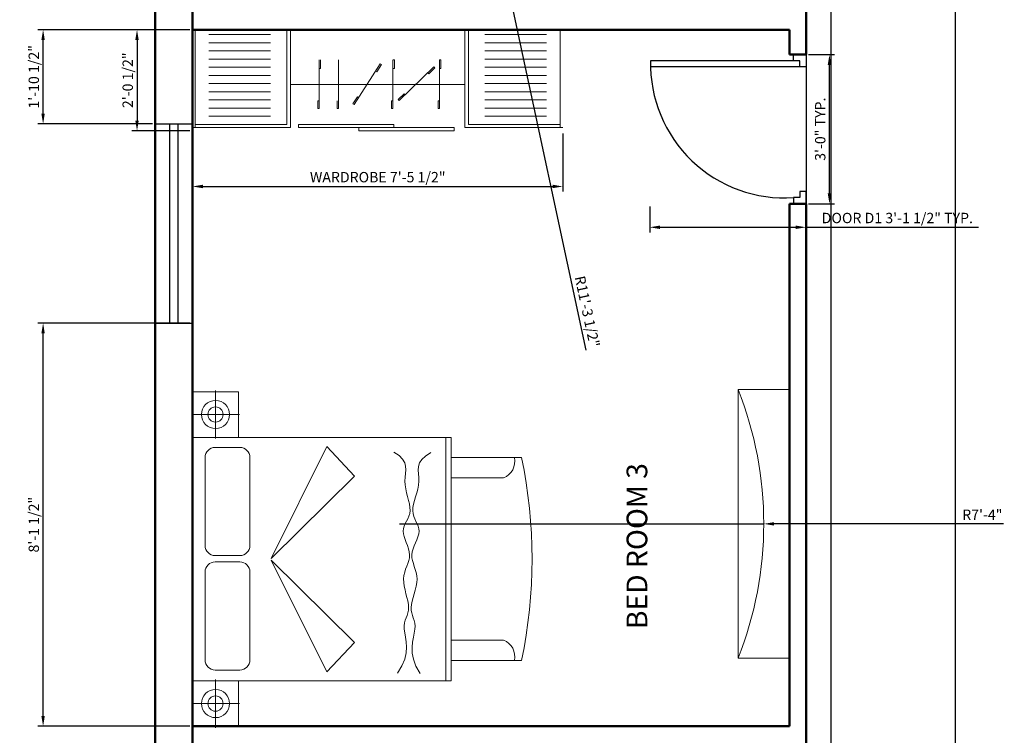
# Model space of a CAD drawing. Units: inches. Extents: x 1905 to 2315, y 3232 to 3824.
# Tile 2 of 8: x 1905 to 2143, y 3442 to 3615. Entities that reach past the tile are written whole.
import ezdxf

# ---------------------------------------------------------------- set-up
doc = ezdxf.new("R2010")
doc.units = ezdxf.units.IN
for name, color, linetype, lineweight in [('A-ANNO-DIMS', 2, 'Continuous', 18), ('A-AREA-IDEN', 7, 'Continuous', 25), ('A-FLOR-CABT', 8, 'Continuous', 18), ('A-FURN', 8, 'Continuous', 18), ('door', 1, 'Continuous', 25), ('TV', 221, 'Continuous', 18), ('wall', 2, 'Continuous', 50), ('WINDOW', 60, 'Continuous', 25)]:
    doc.layers.add(name, color=color, linetype=linetype, lineweight=lineweight)
doc.styles.get("Standard").update_dxf_attribs({"font": 'arial.ttf'})
doc.dimstyles.new('ISO-25', dxfattribs={"dimtxt": 2.5, "dimasz": 2.5, "dimexe": 1.25, "dimexo": 0.625, "dimtad": 1, "dimdec": 1, "dimlunit": 3, "dimtxsty": 'Standard', "dimcen": 2.5, "dimadec": 0, "dimazin": 0, "dimtfac": 1, "dimtdec": 1, "dimtmove": 0, "dimatfit": 3, "dimfxl": 1, "dimarcsym": 0})

# ---------------------------------------------------------------- blocks, each defined once
blk = doc.blocks.new('A$C4F543DC7')
for p, q in [((0.0134, 3.35, -0.1688), (3.3134, 3.35, -0.1688)), ((0.4634, 3.35, -0.1688), (0.0134, 3.35, -0.1688)), ((0.0134, 2.896, -0.1688), (0.0134, 3.35, -0.1688)), ((0.0134, 3.35, -0.1688), (0.0134, 2.896, -0.1688)), ((0.2381, 3.1233, -0.4388), (0.2381, 3.3614, -0.4388)), ((0.4634, 3.35, -0.1688), (0.4634, 0.8, -0.1688)), ((2.8634, 3.35, -0.1688), (0.4634, 3.35, -0.1688)), ((0.4634, 2.896, -0.1688), (0.4634, 3.35, -0.1688)), ((2.8634, 0.8, -0.1688), (2.8634, 3.35, -0.1688)), ((2.8634, 3.35, -0.1688), (3.3134, 3.35, -0.1688)), ((2.8634, 2.896, -0.1688), (2.8634, 3.35, -0.1688)), ((3.0888, 3.1233, -0.4388), (3.0888, 3.3614, -0.4388)), ((3.3134, 3.35, -0.1688), (3.3134, 2.896, -0.1688)), ((3.3134, 3.35, -0.1688), (3.3134, 2.896, -0.1688)), ((1.5354, 3.226, -0.1688), (0.6684, 3.226, -0.1688)), ((2.6644, 3.226, -0.1688), (1.7974, 3.226, -0.1688)), ((0.2381, 3.1233, -0.4388), (0, 3.1233, -0.4388)), ((0.2381, 3.1233, -0.4388), (0.4762, 3.1233, -0.4388)), ((0.2381, 3.1233, -0.4388), (0.2381, 2.8852, -0.4388)), ((0.5684, 3.126, -0.1688), (0.5684, 2.884, -0.1688)), ((1.6354, 2.884, -0.1688), (1.6354, 3.126, -0.1688)), ((1.6974, 3.126, -0.1688), (1.6974, 2.884, -0.1688)), ((2.7644, 2.884, -0.1688), (2.7644, 3.126, -0.1688)), ((3.0888, 3.1233, -0.4388), (2.8507, 3.1233, -0.4388)), ((3.0888, 3.1233, -0.4388), (3.0888, 2.8852, -0.4388)), ((3.0888, 3.1233, -0.4388), (3.3269, 3.1233, -0.4388)), ((0.4634, 2.896, -0.1688), (0.0134, 2.896, -0.1688)), ((0.0134, 2.896, -0.1688), (0.4634, 2.896, -0.1688)), ((0.4634, 0.8, -0.1688), (0.4634, 2.896, -0.1688)), ((2.8634, 2.896, -0.1688), (2.8634, 0.8, -0.1688)), ((3.3134, 2.896, -0.1688), (2.8634, 2.896, -0.1688)), ((3.3134, 2.896, -0.1688), (2.8634, 2.896, -0.1688)), ((0.6684, 2.784, -0.1688), (1.5354, 2.784, -0.1688)), ((1.7974, 2.784, -0.1688), (2.6644, 2.784, -0.1688)), ((1.6534, 2.573, -0.1688), (0.5504, 2.025, -0.1688)), ((0.8414, 1.752, -0.1688), (1.6534, 2.573, -0.1688)), ((2.4814, 1.752, -0.1688), (1.6694, 2.573, -0.1688)), ((1.6694, 2.573, -0.1688), (2.7724, 2.025, -0.1688)), ((0.5504, 2.025, -0.1688), (0.8414, 1.752, -0.1688)), ((2.7724, 2.025, -0.1688), (2.4814, 1.752, -0.1688)), ((2.683, 1.312, -0.1688), (2.7182, 1.3641, -0.1688)), ((0.5369, 1.3267, -0.1688), (0.6088, 1.2835, -0.1688)), ((0.6088, 1.2835, -0.1688), (0.6756, 1.2566, -0.1688)), ((1.3963, 1.2612, -0.1688), (1.4328, 1.2664, -0.1688)), ((1.4328, 1.2664, -0.1688), (1.4679, 1.2677, -0.1688)), ((1.4679, 1.2677, -0.1688), (1.501, 1.2643, -0.1688)), ((1.501, 1.2643, -0.1688), (1.5324, 1.257, -0.1688)), ((1.8557, 1.2531, -0.1688), (1.8849, 1.263, -0.1688)), ((1.8849, 1.263, -0.1688), (1.913, 1.2698, -0.1688)), ((1.913, 1.2698, -0.1688), (1.9397, 1.2722, -0.1688)), ((1.9397, 1.2722, -0.1688), (1.9649, 1.2692, -0.1688)), ((1.9649, 1.2692, -0.1688), (1.989, 1.2617, -0.1688)), ((2.6129, 1.257, -0.1688), (2.6479, 1.2774, -0.1688)), ((2.6479, 1.2774, -0.1688), (2.683, 1.312, -0.1688)), ((0.6067, 1.1458, -0.1688), (0.6743, 1.1706, -0.1688)), ((0.6743, 1.1706, -0.1688), (0.7364, 1.1825, -0.1688)), ((0.6756, 1.2566, -0.1688), (0.7373, 1.2428, -0.1688)), ((0.7364, 1.1825, -0.1688), (0.7931, 1.1846, -0.1688)), ((0.7373, 1.2428, -0.1688), (0.794, 1.239, -0.1688)), ((0.7931, 1.1846, -0.1688), (0.8447, 1.1799, -0.1688)), ((0.794, 1.239, -0.1688), (0.8457, 1.242, -0.1688)), ((0.8447, 1.1799, -0.1688), (0.8913, 1.1716, -0.1688)), ((0.8457, 1.242, -0.1688), (0.8925, 1.2489, -0.1688)), ((0.8913, 1.1716, -0.1688), (0.9331, 1.1628, -0.1688)), ((0.8925, 1.2489, -0.1688), (0.9345, 1.2564, -0.1688)), ((0.9345, 1.2564, -0.1688), (0.9718, 1.2615, -0.1688)), ((0.9718, 1.2615, -0.1688), (1.0044, 1.2617, -0.1688)), ((1.0044, 1.2617, -0.1688), (1.0334, 1.2578, -0.1688)), ((1.0334, 1.2578, -0.1688), (1.0597, 1.2509, -0.1688)), ((1.0583, 1.1642, -0.1688), (1.0831, 1.172, -0.1688)), ((1.0597, 1.2509, -0.1688), (1.0842, 1.2424, -0.1688)), ((1.0831, 1.172, -0.1688), (1.1072, 1.18, -0.1688)), ((1.0842, 1.2424, -0.1688), (1.1081, 1.2336, -0.1688)), ((1.1072, 1.18, -0.1688), (1.1316, 1.1872, -0.1688)), ((1.1081, 1.2336, -0.1688), (1.1322, 1.2257, -0.1688)), ((1.1316, 1.1872, -0.1688), (1.1573, 1.192, -0.1688)), ((1.1322, 1.2257, -0.1688), (1.1577, 1.2201, -0.1688)), ((1.1573, 1.192, -0.1688), (1.1851, 1.1932, -0.1688)), ((1.1577, 1.2201, -0.1688), (1.1855, 1.218, -0.1688)), ((1.1851, 1.1932, -0.1688), (1.2158, 1.1898, -0.1688)), ((1.1855, 1.218, -0.1688), (1.2163, 1.2204, -0.1688)), ((1.2158, 1.1898, -0.1688), (1.2491, 1.1828, -0.1688)), ((1.2163, 1.2204, -0.1688), (1.2498, 1.2264, -0.1688)), ((1.2491, 1.1828, -0.1688), (1.2842, 1.1734, -0.1688)), ((1.2498, 1.2264, -0.1688), (1.2852, 1.2347, -0.1688)), ((1.2842, 1.1734, -0.1688), (1.3206, 1.1629, -0.1688)), ((1.2852, 1.2347, -0.1688), (1.3218, 1.2441, -0.1688)), ((1.3218, 1.2441, -0.1688), (1.3591, 1.2533, -0.1688)), ((1.3591, 1.2533, -0.1688), (1.3963, 1.2612, -0.1688)), ((1.5324, 1.257, -0.1688), (1.5624, 1.2473, -0.1688)), ((1.5624, 1.2473, -0.1688), (1.5915, 1.2365, -0.1688)), ((1.5903, 1.1619, -0.1688), (1.6191, 1.1716, -0.1688)), ((1.5915, 1.2365, -0.1688), (1.6199, 1.2259, -0.1688)), ((1.6191, 1.1716, -0.1688), (1.6475, 1.1797, -0.1688)), ((1.6199, 1.2259, -0.1688), (1.6481, 1.2169, -0.1688)), ((1.6475, 1.1797, -0.1688), (1.676, 1.1849, -0.1688)), ((1.6481, 1.2169, -0.1688), (1.6765, 1.2108, -0.1688)), ((1.676, 1.1849, -0.1688), (1.7049, 1.1858, -0.1688)), ((1.6765, 1.2108, -0.1688), (1.7053, 1.209, -0.1688)), ((1.7049, 1.1858, -0.1688), (1.7344, 1.1816, -0.1688)), ((1.7053, 1.209, -0.1688), (1.7349, 1.2124, -0.1688)), ((1.7344, 1.1816, -0.1688), (1.7643, 1.1731, -0.1688)), ((1.7349, 1.2124, -0.1688), (1.7651, 1.2199, -0.1688)), ((1.7643, 1.1731, -0.1688), (1.7944, 1.1619, -0.1688)), ((1.7651, 1.2199, -0.1688), (1.7955, 1.2301, -0.1688)), ((1.7955, 1.2301, -0.1688), (1.8258, 1.2417, -0.1688)), ((1.8258, 1.2417, -0.1688), (1.8557, 1.2531, -0.1688)), ((1.989, 1.2617, -0.1688), (2.0124, 1.2512, -0.1688)), ((2.0124, 1.2512, -0.1688), (2.0359, 1.2391, -0.1688)), ((2.0359, 1.2391, -0.1688), (2.0599, 1.2269, -0.1688)), ((2.0588, 1.1568, -0.1688), (2.0842, 1.167, -0.1688)), ((2.0599, 1.2269, -0.1688), (2.0849, 1.216, -0.1688)), ((2.0842, 1.167, -0.1688), (2.1112, 1.1743, -0.1688)), ((2.0849, 1.216, -0.1688), (2.1117, 1.2077, -0.1688)), ((2.1112, 1.1743, -0.1688), (2.1403, 1.1775, -0.1688)), ((2.1117, 1.2077, -0.1688), (2.1407, 1.2037, -0.1688)), ((2.1403, 1.1775, -0.1688), (2.1718, 1.1755, -0.1688)), ((2.1407, 1.2037, -0.1688), (2.1723, 1.2047, -0.1688)), ((2.1718, 1.1755, -0.1688), (2.2056, 1.1691, -0.1688)), ((2.1723, 1.2047, -0.1688), (2.2062, 1.21, -0.1688)), ((2.2056, 1.1691, -0.1688), (2.2411, 1.1598, -0.1688)), ((2.2062, 1.21, -0.1688), (2.242, 1.2182, -0.1688)), ((2.242, 1.2182, -0.1688), (2.2791, 1.2279, -0.1688)), ((2.2791, 1.2279, -0.1688), (2.3173, 1.2378, -0.1688)), ((2.3173, 1.2378, -0.1688), (2.3558, 1.2465, -0.1688)), ((2.3558, 1.2465, -0.1688), (2.3944, 1.2527, -0.1688)), ((2.3944, 1.2527, -0.1688), (2.4325, 1.255, -0.1688)), ((2.4325, 1.255, -0.1688), (2.4698, 1.2529, -0.1688)), ((2.4698, 1.2529, -0.1688), (2.5064, 1.2488, -0.1688)), ((2.5064, 1.2488, -0.1688), (2.5423, 1.2459, -0.1688)), ((2.5423, 1.2459, -0.1688), (2.5777, 1.2476, -0.1688)), ((2.5777, 1.2476, -0.1688), (2.6129, 1.257, -0.1688)), ((0.5334, 1.105, -0.1688), (0.6067, 1.1458, -0.1688)), ((0.9331, 1.1628, -0.1688), (0.9701, 1.1565, -0.1688)), ((0.9701, 1.1565, -0.1688), (1.0027, 1.1552, -0.1688)), ((1.0027, 1.1552, -0.1688), (1.0318, 1.1582, -0.1688)), ((1.0318, 1.1582, -0.1688), (1.0583, 1.1642, -0.1688)), ((1.3206, 1.1629, -0.1688), (1.3575, 1.1524, -0.1688)), ((1.3575, 1.1524, -0.1688), (1.3945, 1.1434, -0.1688)), ((1.3945, 1.1434, -0.1688), (1.4308, 1.1371, -0.1688)), ((1.4308, 1.1371, -0.1688), (1.4658, 1.1347, -0.1688)), ((1.4658, 1.1347, -0.1688), (1.499, 1.137, -0.1688)), ((1.499, 1.137, -0.1688), (1.5306, 1.1433, -0.1688)), ((1.5306, 1.1433, -0.1688), (1.5609, 1.152, -0.1688)), ((1.5609, 1.152, -0.1688), (1.5903, 1.1619, -0.1688)), ((1.7944, 1.1619, -0.1688), (1.8244, 1.1494, -0.1688)), ((1.8244, 1.1494, -0.1688), (1.8539, 1.137, -0.1688)), ((1.8539, 1.137, -0.1688), (1.8827, 1.1263, -0.1688)), ((1.8827, 1.1263, -0.1688), (1.9106, 1.1186, -0.1688)), ((1.9106, 1.1186, -0.1688), (1.9373, 1.1153, -0.1688)), ((1.9373, 1.1153, -0.1688), (1.9625, 1.1176, -0.1688)), ((1.9625, 1.1176, -0.1688), (1.9868, 1.1243, -0.1688)), ((1.9868, 1.1243, -0.1688), (2.0106, 1.134, -0.1688)), ((2.0106, 1.134, -0.1688), (2.0344, 1.1454, -0.1688)), ((2.0344, 1.1454, -0.1688), (2.0588, 1.1568, -0.1688)), ((2.2411, 1.1598, -0.1688), (2.2779, 1.1489, -0.1688)), ((2.2779, 1.1489, -0.1688), (2.3157, 1.1379, -0.1688)), ((2.3157, 1.1379, -0.1688), (2.354, 1.1279, -0.1688)), ((2.354, 1.1279, -0.1688), (2.3923, 1.1205, -0.1688)), ((2.3923, 1.1205, -0.1688), (2.4304, 1.117, -0.1688)), ((2.4304, 1.117, -0.1688), (2.4677, 1.118, -0.1688)), ((2.4677, 1.118, -0.1688), (2.5043, 1.1209, -0.1688)), ((2.5043, 1.1209, -0.1688), (2.5403, 1.1226, -0.1688)), ((2.5403, 1.1226, -0.1688), (2.5757, 1.1199, -0.1688)), ((2.5757, 1.1199, -0.1688), (2.6106, 1.1094, -0.1688)), ((2.6106, 1.1094, -0.1688), (2.645, 1.0879, -0.1688)), ((2.645, 1.0879, -0.1688), (2.6789, 1.0522, -0.1688)), ((2.6789, 1.0522, -0.1688), (2.7124, 0.999, -0.1688)), ((0.4634, 0.85, -0.1688), (2.8634, 0.85, -0.1688)), ((0.4634, 0.8, -0.1688), (2.8634, 0.8, -0.1688)), ((0.6634, 0.8, -0.1688), (0.4634, 0.8, -0.1688)), ((0.6634, 0.8, -0.1688), (2.6634, 0.8, -0.1688)), ((0.6634, 0.104, -0.1688), (0.6634, 0.8, -0.1688)), ((0.6634, 0.104, -0.1688), (0.6634, 0.8, -0.1688)), ((0.8634, 0.281, -0.1688), (0.8634, 0.8, -0.1688)), ((2.4634, 0.8, -0.1688), (2.4634, 0.281, -0.1688)), ((2.8634, 0.8, -0.1688), (2.6634, 0.8, -0.1688)), ((2.6634, 0.8, -0.1688), (2.6634, 0.104, -0.1688)), ((2.6634, 0.8, -0.1688), (2.6634, 0.104, -0.1688))]:
    blk.add_line(p, q)
for centre, radius in [((0.2381, 3.1233, -0.4388), 0.139), ((3.0888, 3.1233, -0.4388), 0.139), ((0.2381, 3.1233, -0.4388), 0.075), ((3.0888, 3.1233, -0.4388), 0.075)]:
    blk.add_circle(centre, radius)
for centre, radius, start, end in [((0.6684, 3.126, -0.1688), 0.1, 90, 180), ((1.5354, 3.126, -0.1688), 0.1, 0, 90), ((1.7974, 3.126, -0.1688), 0.1, 90, 180), ((2.6644, 3.126, -0.1688), 0.1, 0, 90), ((0.6684, 2.884, -0.1688), 0.1, 180, 270), ((1.5354, 2.884, -0.1688), 0.1, 270, 0), ((1.7974, 2.884, -0.1688), 0.1, 180, 270), ((2.6644, 2.884, -0.1688), 0.1, 270, 0), ((0.6994, 0.3472, -0.1688), 0.1769, 258.2616, 338.03196), ((2.6275, 0.3472, -0.1688), 0.1769, 201.96804, 281.7384), ((1.6634, 4.8597, -0.1688), 4.8597, 258.12517, 281.87483), ((1.6634, 4.8597, -0.1688), 4.8597, 258.12517, 281.87483)]:
    blk.add_arc(centre, radius, start, end)
blk = doc.blocks.new('A$C34930FF8')
at = {"ltscale": 0.05}
for p, q in [((0, 2252.4), (0, 16.8)), ((600, 2252.4), (0, 2252.4)), ((185.4, 1513), (185.4, 1521.5)), ((237.7, 1513), (237.7, 1521.5)), ((436.7, 1513), (436.7, 1504.4)), ((482.5, 1513), (482.5, 1504.4)), ((227.1, 1479.2), (233.2, 1485.2)), ((263.6, 1441.7), (269.7, 1447.7)), ((398.2, 1303.6), (392.1, 1297.6)), ((185.4, 1229.1), (185.4, 1237.7)), ((237.7, 1229.1), (237.7, 1237.7)), ((434.8, 1266.1), (428.7, 1260.1)), ((436.7, 1228.2), (436.7, 1219.7)), ((482.5, 1228.2), (482.5, 1219.7)), ((209.5, 1150.1), (214.1, 1157.3)), ((253.5, 1121.8), (258.1, 1129)), ((415.3, 1017.6), (410.6, 1010.5)), ((459.3, 989.3), (454.7, 982.1)), ((482.5, 894.9), (482.5, 886.3)), ((237.7, 775.3), (237.7, 783.9)), ((436.7, 775.3), (436.7, 766.8)), ((482.5, 775.3), (482.5, 766.8)), ((600, 16.8), (0, 16.8))]:
    blk.add_line(p, q, dxfattribs=at)
for p, q in [((580, 1690.9), (580, 2252.4)), ((600, 1669.3), (600, 2269.3)), ((30, 1790.9), (30, 2169.3)), ((80, 1790.9), (80, 2169.3)), ((130, 1790.9), (130, 2169.3)), ((180, 1790.9), (180, 2169.3)), ((230, 1790.9), (230, 2169.3)), ((280, 1790.9), (280, 2169.3)), ((330, 1790.9), (330, 2169.3)), ((380, 1790.9), (380, 2169.3)), ((430, 1790.9), (430, 2169.3)), ((480, 1790.9), (480, 2169.3)), ((530, 1790.9), (530, 2169.3)), ((580, 1690.9), (0, 1690.9)), ((600, 1669.3), (0, 1669.3)), ((335.4, 1666.1), (335.4, 603.1)), ((600, 1603.3), (620, 1603.3)), ((600, 1018.7), (600, 1603.3)), ((620, 1603.3), (620, 1018.7)), ((237.7, 1521.5), (185.4, 1521.5)), ((482.5, 1513), (185.4, 1513)), ((434.8, 1266.1), (227.4, 1478.9)), ((269.7, 1447.7), (233.2, 1485.2)), ((436.7, 1504.4), (482.5, 1504.4)), ((428.7, 1260.1), (392.1, 1297.6)), ((237.7, 1237.7), (185.4, 1237.7)), ((482.5, 1228.2), (185.4, 1228.2)), ((436.7, 1219.7), (482.5, 1219.7)), ((600, 1233.4), (580, 1233.4)), ((580, 1233.4), (580, 648.7)), ((600, 648.7), (600, 1233.4)), ((459.3, 989.3), (209.5, 1150.1)), ((258.1, 1129), (214.1, 1157.3)), ((454.7, 982.1), (410.6, 1010.5)), ((620, 1018.7), (600, 1018.7)), ((482.5, 894.9), (185.4, 894.9)), ((436.7, 886.3), (482.5, 886.3)), ((237.7, 783.9), (185.4, 783.9)), ((482.5, 775.3), (185.4, 775.3)), ((436.7, 766.8), (482.5, 766.8)), ((580, 648.7), (600, 648.7)), ((600, 600), (0, 600)), ((580, 578.3), (0, 578.3)), ((580, 578.3), (580, 16.8)), ((600, 600), (600, 0)), ((30, 478.3), (30, 100)), ((80, 478.3), (80, 100)), ((130, 478.3), (130, 100)), ((180, 478.3), (180, 100)), ((230, 478.3), (230, 100)), ((280, 478.3), (280, 100)), ((330, 478.3), (330, 100)), ((380, 478.3), (380, 100)), ((430, 478.3), (430, 100)), ((480, 478.3), (480, 100)), ((530, 478.3), (530, 100))]:
    blk.add_line(p, q)
blk = doc.blocks.new('DOOR-SWING-36IN')
for p, q in [((34.51, 36), (37.51, 36)), ((34.51, 34.5), (34.51, 36)), ((37.51, 36), (37.51, 33)), ((36.01, 34.5), (0.01, 34.5)), ((36.01, 34.5), (34.51, 34.5)), ((36.01, 33), (36.01, 34.5)), ((36.01, 33), (0.01, 33)), ((37.51, 33), (36.01, 33)), ((37.51, 3), (36.01, 3)), ((36.01, 3), (36.01, 1.5)), ((37.51, 0), (37.51, 3)), ((36.01, 1.5), (34.51, 1.5)), ((34.51, 1.5), (34.51, 0)), ((34.51, 0), (37.51, 0))]:
    blk.add_line(p, q)
blk.add_arc((32.32, 33.75), 32.32, 178.6705, 273.8756)
blk = doc.blocks.new('WIN-48IN')
for p, q in [((0, 9), (0, 0)), ((0, 9), (48, 9)), ((48, 9), (48, 0)), ((0, 5.5), (48, 5.5)), ((0, 3.5), (48, 3.5)), ((0, 0), (48, 0))]:
    blk.add_line(p, q)
blk = doc.blocks.new('*D25')
at = {"layer": 'A-ANNO-DIMS', "color": 0, "lineweight": -2, "transparency": 16777216}
for p, q in [((2057.3, 3569.61), (2057.3, 3563.33)), ((2095.01, 3569.61), (2095.01, 3563.33)), ((2059.8, 3564.58), (2092.51, 3564.58)), ((2095.01, 3564.58), (2136.58, 3564.58))]:
    blk.add_line(p, q, dxfattribs=at)
at = {"layer": 'A-ANNO-DIMS', "color": 0, "transparency": 16777216}
for points in [[(2059.8, 3564.99), (2059.8, 3564.16), (2057.3, 3564.58)], [(2092.51, 3564.99), (2092.51, 3564.16), (2095.01, 3564.58)]]:
    blk.add_solid(points, dxfattribs=at)
at = {"layer": 'Defpoints', "color": 0, "transparency": 16777216}
for p in [(2057.3, 3570.23), (2095.01, 3570.23), (2095.01, 3564.58)]:
    blk.add_point(p, dxfattribs=at)
at = {"layer": 'A-ANNO-DIMS', "color": 0, "transparency": 16777216, "insert": (2117.04, 3566.49), "char_height": 2.5, "attachment_point": 5}
blk.add_mtext('DOOR D1 3\'-1 1/2" TYP.', dxfattribs=at)
blk = doc.blocks.new('*D26')
at = {"layer": 'A-ANNO-DIMS', "color": 0, "lineweight": -2, "transparency": 16777216}
for p, q in [((2095.63, 3606.23), (2101.91, 3606.23)), ((2100.66, 3572.73), (2100.66, 3603.73)), ((2095.63, 3570.23), (2101.91, 3570.23))]:
    blk.add_line(p, q, dxfattribs=at)
at = {"layer": 'A-ANNO-DIMS', "color": 0, "transparency": 16777216}
for points in [[(2100.25, 3603.73), (2101.08, 3603.73), (2100.66, 3606.23)], [(2100.25, 3572.73), (2101.08, 3572.73), (2100.66, 3570.23)]]:
    blk.add_solid(points, dxfattribs=at)
at = {"layer": 'Defpoints', "color": 0, "transparency": 16777216}
for p in [(2095.01, 3606.23), (2100.66, 3606.23), (2095.01, 3570.23)]:
    blk.add_point(p, dxfattribs=at)
at = {"layer": 'A-ANNO-DIMS', "color": 0, "transparency": 16777216, "insert": (2098.76, 3588.23), "char_height": 2.5, "attachment_point": 5, "rotation": 90}
blk.add_mtext('3\'-0" TYP.', dxfattribs=at)
blk = doc.blocks.new('*D31')
at = {"layer": 'A-ANNO-DIMS', "color": 0, "lineweight": -2, "transparency": 16777216}
for p, q in [((1947.01, 3587.2), (1947.01, 3573.17)), ((2036.35, 3587.2), (2036.35, 3573.17)), ((1949.51, 3574.42), (2033.85, 3574.42))]:
    blk.add_line(p, q, dxfattribs=at)
at = {"layer": 'A-ANNO-DIMS', "color": 0, "transparency": 16777216}
for points in [[(1949.51, 3574.84), (1949.51, 3574), (1947.01, 3574.42)], [(2033.85, 3574.84), (2033.85, 3574), (2036.35, 3574.42)]]:
    blk.add_solid(points, dxfattribs=at)
at = {"layer": 'Defpoints', "color": 0, "transparency": 16777216}
for p in [(1947.01, 3587.82), (2036.35, 3587.82), (2036.35, 3574.42)]:
    blk.add_point(p, dxfattribs=at)
at = {"layer": 'A-ANNO-DIMS', "color": 0, "transparency": 16777216, "insert": (1991.68, 3576.34), "char_height": 2.5, "attachment_point": 5}
blk.add_mtext('WARDROBE 7\'-5 1/2"', dxfattribs=at)
blk = doc.blocks.new('*D32')
at = {"layer": 'A-ANNO-DIMS', "color": 0, "lineweight": -2, "transparency": 16777216}
for p, q in [((1946.38, 3612.23), (1932.36, 3612.23)), ((1933.61, 3609.73), (1933.61, 3590.32)), ((1946.38, 3587.82), (1932.36, 3587.82))]:
    blk.add_line(p, q, dxfattribs=at)
at = {"layer": 'A-ANNO-DIMS', "color": 0, "transparency": 16777216}
for points in [[(1933.19, 3609.73), (1934.02, 3609.73), (1933.61, 3612.23)], [(1933.19, 3590.32), (1934.02, 3590.32), (1933.61, 3587.82)]]:
    blk.add_solid(points, dxfattribs=at)
at = {"layer": 'Defpoints', "color": 0, "transparency": 16777216}
for p in [(1947.01, 3612.23), (1933.61, 3587.82), (1947.01, 3587.82)]:
    blk.add_point(p, dxfattribs=at)
at = {"layer": 'A-ANNO-DIMS', "color": 0, "transparency": 16777216, "insert": (1931.69, 3600.03), "char_height": 2.5, "attachment_point": 5, "rotation": 90}
blk.add_mtext('2\'-0 1/2"', dxfattribs=at)
blk = doc.blocks.new('*D41')
at = {"layer": 'A-ANNO-DIMS', "color": 0, "lineweight": -2, "transparency": 16777216}
for p, q in [((2095.01, 3663.61), (2095.01, 3232.16)), ((2171.01, 3663.61), (2171.01, 3232.16)), ((2097.51, 3233.41), (2168.51, 3233.41))]:
    blk.add_line(p, q, dxfattribs=at)
at = {"layer": 'A-ANNO-DIMS', "color": 0, "transparency": 16777216}
for points in [[(2097.51, 3233.83), (2097.51, 3233), (2095.01, 3233.41)], [(2168.51, 3233.83), (2168.51, 3233), (2171.01, 3233.41)]]:
    blk.add_solid(points, dxfattribs=at)
at = {"layer": 'Defpoints', "color": 0, "transparency": 16777216}
for p in [(2095.01, 3664.23), (2171.01, 3664.23), (2171.01, 3233.41)]:
    blk.add_point(p, dxfattribs=at)
at = {"layer": 'A-ANNO-DIMS', "color": 0, "transparency": 16777216, "insert": (2133.01, 3235.31), "char_height": 2.5, "attachment_point": 5}
blk.add_mtext('6\'-4"', dxfattribs=at)
blk = doc.blocks.new('*D46')
at = {"layer": 'A-ANNO-DIMS', "color": 0, "lineweight": -2, "transparency": 16777216}
for p, q in [((1946.38, 3541.49), (1909.7, 3541.49)), ((1910.95, 3446.73), (1910.95, 3538.99)), ((1946.38, 3444.23), (1909.7, 3444.23))]:
    blk.add_line(p, q, dxfattribs=at)
at = {"layer": 'A-ANNO-DIMS', "color": 0, "transparency": 16777216}
for points in [[(1910.53, 3538.99), (1911.36, 3538.99), (1910.95, 3541.49)], [(1910.53, 3446.73), (1911.36, 3446.73), (1910.95, 3444.23)]]:
    blk.add_solid(points, dxfattribs=at)
at = {"layer": 'Defpoints', "color": 0, "transparency": 16777216}
for p in [(1910.95, 3541.49), (1947.01, 3541.49), (1947.01, 3444.23)]:
    blk.add_point(p, dxfattribs=at)
at = {"layer": 'A-ANNO-DIMS', "color": 0, "transparency": 16777216, "insert": (1909.03, 3492.86), "char_height": 2.5, "attachment_point": 5, "rotation": 90}
blk.add_mtext('8\'-1 1/2"', dxfattribs=at)
blk = doc.blocks.new('*D47')
at = {"layer": 'A-ANNO-DIMS', "color": 0, "lineweight": -2, "transparency": 16777216}
for p, q in [((1946.38, 3612.23), (1909.7, 3612.23)), ((1910.95, 3591.99), (1910.95, 3609.73)), ((1937.38, 3589.49), (1909.7, 3589.49))]:
    blk.add_line(p, q, dxfattribs=at)
at = {"layer": 'A-ANNO-DIMS', "color": 0, "transparency": 16777216}
for points in [[(1910.53, 3609.73), (1911.36, 3609.73), (1910.95, 3612.23)], [(1910.53, 3591.99), (1911.36, 3591.99), (1910.95, 3589.49)]]:
    blk.add_solid(points, dxfattribs=at)
at = {"layer": 'Defpoints', "color": 0, "transparency": 16777216}
for p in [(1910.95, 3612.23), (1947.01, 3612.23), (1938.01, 3589.49)]:
    blk.add_point(p, dxfattribs=at)
at = {"layer": 'A-ANNO-DIMS', "color": 0, "transparency": 16777216, "insert": (1909.03, 3600.86), "char_height": 2.5, "attachment_point": 5, "rotation": 90}
blk.add_mtext('1\'-10 1/2"', dxfattribs=at)
blk = doc.blocks.new('*D64')
at = {"layer": 'A-ANNO-DIMS', "color": 0, "lineweight": -2, "transparency": 16777216}
for p, q in [((2101.01, 3659.61), (2101.01, 3232.16)), ((2131.01, 3659.61), (2131.01, 3232.16)), ((2103.51, 3233.41), (2128.51, 3233.41))]:
    blk.add_line(p, q, dxfattribs=at)
at = {"layer": 'A-ANNO-DIMS', "color": 0, "transparency": 16777216}
for points in [[(2103.51, 3233.83), (2103.51, 3233), (2101.01, 3233.41)], [(2128.51, 3233.83), (2128.51, 3233), (2131.01, 3233.41)]]:
    blk.add_solid(points, dxfattribs=at)
at = {"layer": 'Defpoints', "color": 0, "transparency": 16777216}
for p in [(2101.01, 3660.23), (2131.01, 3660.23), (2131.01, 3233.41)]:
    blk.add_point(p, dxfattribs=at)
at = {"layer": 'A-ANNO-DIMS', "color": 0, "transparency": 16777216, "insert": (2116.01, 3235.31), "char_height": 2.5, "attachment_point": 5}
blk.add_mtext('2\'-6"', dxfattribs=at)
blk = doc.blocks.new('*D65')
at = {"layer": 'A-ANNO-DIMS', "color": 0, "lineweight": -2, "transparency": 16777216}
for p, q in [((2095.01, 3659.61), (2095.01, 3232.16)), ((2101.01, 3659.61), (2101.01, 3232.16)), ((2092.51, 3233.41), (2090.01, 3233.41)), ((2095.01, 3233.41), (2101.01, 3233.41)), ((2103.51, 3233.41), (2113.9, 3233.41))]:
    blk.add_line(p, q, dxfattribs=at)
at = {"layer": 'A-ANNO-DIMS', "color": 0, "transparency": 16777216}
for points in [[(2092.51, 3233.83), (2092.51, 3233), (2095.01, 3233.41)], [(2103.51, 3233.83), (2103.51, 3233), (2101.01, 3233.41)]]:
    blk.add_solid(points, dxfattribs=at)
at = {"layer": 'Defpoints', "color": 0, "transparency": 16777216}
for p in [(2095.01, 3660.23), (2101.01, 3660.23), (2101.01, 3233.41)]:
    blk.add_point(p, dxfattribs=at)
at = {"layer": 'A-ANNO-DIMS', "color": 0, "transparency": 16777216, "insert": (2109.96, 3235.31), "char_height": 2.5, "attachment_point": 5}
blk.add_mtext('0\'-6"', dxfattribs=at)
blk = doc.blocks.new('*D77')
at = {"layer": 'A-ANNO-DIMS', "color": 0, "lineweight": -2, "transparency": 16777216}
for p, q in [((1994.59, 3755.82), (2023, 3623.3)), ((2041.94, 3534.97), (2023.52, 3620.86))]:
    blk.add_line(p, q, dxfattribs=at)
at = {"layer": 'A-ANNO-DIMS', "color": 0, "transparency": 16777216}
blk.add_solid([(2023.93, 3620.95), (2023.12, 3620.77), (2023, 3623.3)], dxfattribs=at)
at = {"layer": 'Defpoints', "color": 0, "transparency": 16777216}
for p in [(1994.59, 3755.82), (2023, 3623.3)]:
    blk.add_point(p, dxfattribs=at)
at = {"layer": 'A-ANNO-DIMS', "color": 0, "transparency": 16777216, "insert": (2041.92, 3544.2), "char_height": 2.5, "attachment_point": 5, "rotation": 282.0988}
blk.add_mtext('R11\'-3 1/2"', dxfattribs=at)
blk = doc.blocks.new('*D78')
at = {"layer": 'A-ANNO-DIMS', "color": 0, "lineweight": -2, "transparency": 16777216}
for p, q in [((1996.94, 3493.06), (2084.82, 3493.06)), ((2142.68, 3493.06), (2087.32, 3493.06))]:
    blk.add_line(p, q, dxfattribs=at)
at = {"layer": 'A-ANNO-DIMS', "color": 0, "transparency": 16777216}
blk.add_solid([(2087.32, 3493.47), (2087.32, 3492.64), (2084.82, 3493.06)], dxfattribs=at)
at = {"layer": 'Defpoints', "color": 0, "transparency": 16777216}
for p in [(1996.94, 3493.06), (2084.82, 3493.06)]:
    blk.add_point(p, dxfattribs=at)
at = {"layer": 'A-ANNO-DIMS', "color": 0, "transparency": 16777216, "insert": (2137.54, 3494.93), "char_height": 2.5, "attachment_point": 5, "rotation": 0.0002}
blk.add_mtext('R7\'-4"', dxfattribs=at)

msp = doc.modelspace()

# ---------------------------------------------------------------- linework, layer by layer
at = {"layer": 'TV'}
msp.add_lwpolyline([(2091.01, 3525.46), (2078.62, 3525.46), (2078.62, 3460.66), (2091.01, 3460.66)], close=True, dxfattribs=at)
msp.add_arc((1996.94, 3493.06), 87.87, 338.3635, 21.6365, dxfattribs=at)
at = {"layer": 'wall'}
for p, q in [((1938.01, 3793.23), (1938.01, 3277.23)), ((1947.01, 3784.23), (1947.01, 3286.23)), ((2095.01, 3622.23), (2095.01, 3606.23)), ((2091.01, 3612.23), (1947.01, 3612.23)), ((2091.01, 3612.23), (2091.01, 3606.23)), ((2091.01, 3606.23), (2095.01, 3606.23)), ((2091.01, 3570.23), (2095.01, 3570.23)), ((2091.01, 3570.23), (2091.01, 3444.23)), ((2095.01, 3570.23), (2095.01, 3434.23)), ((2091.01, 3444.23), (1947.01, 3444.23))]:
    msp.add_line(p, q, dxfattribs=at)

# ---------------------------------------------------------------- block references
at = {"layer": 'A-FLOR-CABT', "xscale": 0.0393700787401575, "yscale": 0.0393700787401575, "zscale": 0.0393700787401575, "rotation": 270}
msp.add_blockref('A$C34930FF8', (1947.01, 3612.23), dxfattribs=at)
at = {"layer": 'A-FURN', "xscale": 24.45263891714, "yscale": 24.45263891714, "zscale": 24.45263891714, "rotation": 90}
msp.add_blockref('A$C4F543DC7', (2028.92, 3443.9, 4.13), dxfattribs=at)
at = {"layer": 'door'}
msp.add_blockref('DOOR-SWING-36IN', (2057.5, 3570.23), dxfattribs=at)
at = {"layer": 'WINDOW', "rotation": 89.99999999999793}
msp.add_blockref('WIN-48IN', (1947.01, 3541.49), dxfattribs=at)

# ---------------------------------------------------------------- texts
at = {"layer": 'A-AREA-IDEN', "insert": (2051.72, 3467.68), "char_height": 5, "attachment_point": 1, "rotation": 90}
msp.add_mtext_dynamic_manual_height_columns('BED ROOM 3', width=56.1502, gutter_width=12.5, heights=[0], dxfattribs=at)

# ---------------------------------------------------------------- dimensions: what is measured, and where the dimension line sits
at = {"layer": 'A-ANNO-DIMS'}
for center, mpoint, picture, middle in [((1994.59, 3755.82), (2023, 3623.3), '*D77', (2040.04, 3543.79)), ((1996.94, 3493.06), (2084.82, 3493.06), '*D78', (2137.54, 3493.06))]:
    dim = msp.add_radius_dim(center=center, mpoint=mpoint, dimstyle='ISO-25', override={"dimdec": 1, "dimlfac": 1, "dimrnd": 0, "dimzin": 1, "dimdsep": 46, "dimlunit": 4, "dimfrac": 2}, dxfattribs=at)
    dim.commit()
    dim.dimension.update_dxf_attribs({"geometry": picture, "text_midpoint": middle, "dimtype": 164})
for base, p1, p2, picture, middle in [((2171.01, 3233.41), (2095.01, 3664.23), (2171.01, 3664.23), '*D41', (2133.01, 3235.31)), ((2101.01, 3233.41), (2095.01, 3660.23), (2101.01, 3660.23), '*D65', (2109.96, 3235.31)), ((2131.01, 3233.41), (2101.01, 3660.23), (2131.01, 3660.23), '*D64', (2116.01, 3235.31))]:
    dim = msp.add_linear_dim(base=base, p1=p1, p2=p2, dimstyle='ISO-25', override={"dimdec": 1, "dimlfac": 1, "dimrnd": 0, "dimzin": 1, "dimdsep": 46, "dimlunit": 4, "dimfrac": 2}, dxfattribs=at)
    dim.commit()
    dim.dimension.update_dxf_attribs({"geometry": picture, "text_midpoint": middle})
for base, p1, p2, angle, picture, middle in [((1910.95, 3612.23), (1938.01, 3589.49), (1947.01, 3612.23), 90, '*D47', (1909.03, 3600.86)), ((1933.61, 3587.82), (1947.01, 3612.23), (1947.01, 3587.82), 270, '*D32', (1931.69, 3600.03)), ((1910.95, 3541.49), (1947.01, 3444.23), (1947.01, 3541.49), 90, '*D46', (1909.03, 3492.86))]:
    dim = msp.add_linear_dim(base=base, p1=p1, p2=p2, angle=angle, dimstyle='ISO-25', override={"dimdec": 1, "dimlfac": 1, "dimrnd": 0, "dimzin": 1, "dimdsep": 46, "dimlunit": 4, "dimfrac": 2}, dxfattribs=at)
    dim.commit()
    dim.dimension.update_dxf_attribs({"geometry": picture, "text_midpoint": middle})
dim = msp.add_linear_dim(base=(2100.66, 3606.23), p1=(2095.01, 3570.23), p2=(2095.01, 3606.23), angle=90, text='<> TYP.', dimstyle='ISO-25', override={"dimdec": 1, "dimlfac": 1, "dimrnd": 0, "dimzin": 1, "dimdsep": 46, "dimlunit": 4, "dimfrac": 2}, dxfattribs=at)
dim.commit()
dim.dimension.update_dxf_attribs({"geometry": '*D26', "text_midpoint": (2098.76, 3588.23)})
for base, p1, p2, text, picture, middle in [((2036.35, 3574.42), (1947.01, 3587.82), (2036.35, 3587.82), 'WARDROBE <>', '*D31', (1991.68, 3576.34)), ((2095.01, 3564.58), (2057.3, 3570.23), (2095.01, 3570.23), 'DOOR D1 <> TYP.', '*D25', (2117.04, 3566.49))]:
    dim = msp.add_linear_dim(base=base, p1=p1, p2=p2, text=text, dimstyle='ISO-25', override={"dimdec": 1, "dimlfac": 1, "dimrnd": 0, "dimzin": 1, "dimdsep": 46, "dimlunit": 4, "dimfrac": 2}, dxfattribs=at)
    dim.commit()
    dim.dimension.update_dxf_attribs({"geometry": picture, "text_midpoint": middle})

doc.saveas('drawing.dxf')
